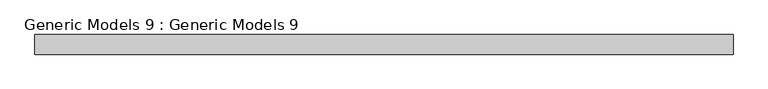
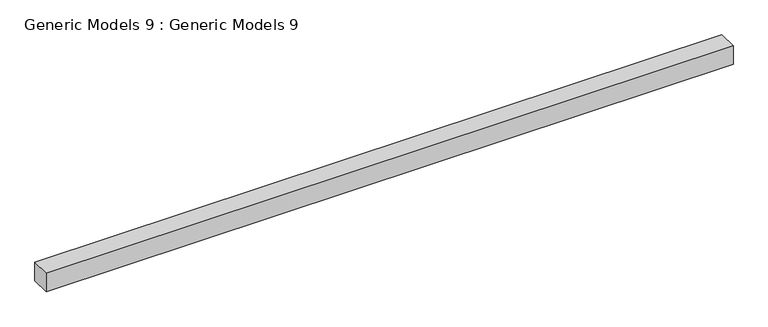
"""IFC4 building model written with IfcOpenShell, lengths in millimetres: proxy geometry, Generic Models 9 : Generic Models 9."""

from ifc_helpers import new_model, si_unit, frame, origin, place, context, project, spatial, polyline, outline, extrude, source, transform, mapped, element, save


def generic_models_9_generic_models_9_b7a25faa(model_context):
    return source(origin(), model_context, "Body", "SweptSolid", [
        extrude(outline(polyline([(3157.8883646, -21302.9985361), (-7701.088074, -21302.9985361), (-7701.088074, -20998.1985361), (3157.8883646, -20998.1985361), (3157.8883646, -21302.9985361)])), frame((0.0, 0.0, 12801.6), z_axis=(0.0, 0.0, 1.0), x_axis=(1.0, 0.0, 0.0)), (0.0, 0.0, 1.0), 304.8),
    ])


if __name__ == "__main__":
    model = new_model("IFC4")
    model_context = context("Model", 3, world=origin())
    ifc_project = project(units=[si_unit("LENGTHUNIT", "METRE", prefix="MILLI")], contexts=[model_context])
    site = spatial("IfcSite", under=ifc_project)
    building = spatial("IfcBuilding", under=site)
    placement = place(None, origin())
    generic_models_9_generic_models_9_shape = generic_models_9_generic_models_9_b7a25faa(model_context)
    element("IfcBuildingElementProxy", 1, Name="Generic Models 9 : Generic Models 9", ObjectType="Generic Models 9 : Generic Models 9", at=placement, inside=building, context=model_context, shape_type="MappedRepresentation", body=[
        mapped(generic_models_9_generic_models_9_shape, transform((0.0, 0.0, 0.0), x_axis=(1.0, 0.0, 0.0), y_axis=(0.0, 1.0, 0.0), z_axis=(0.0, 0.0, 1.0))),
    ])
    save(model, "model.ifc")
